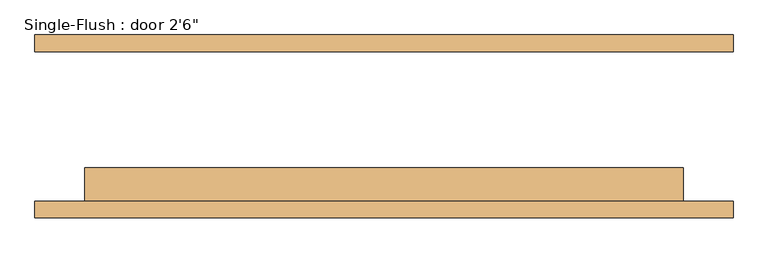
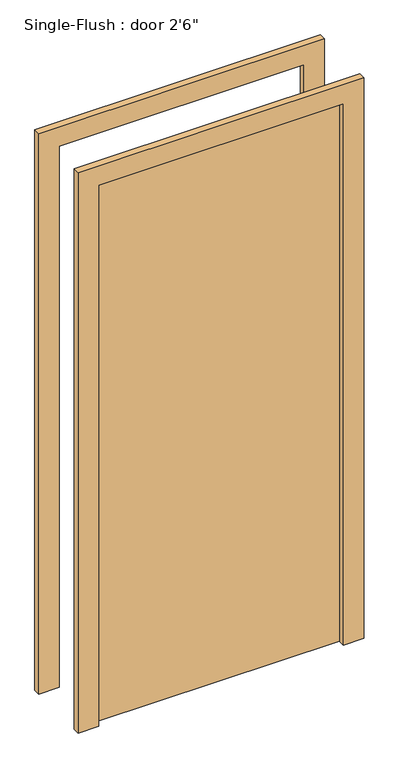
"""IFC4 building model written with IfcOpenShell, lengths in millimetres: door geometry."""

from ifc_helpers import new_model, si_unit, frame, origin, origin_with_axes, place, context, project, spatial, polyline, outline, extrude, source, transform, mapped, element, save


def door_a90ba1ad(model_context):
    return source(origin(), model_context, "Body", "SweptSolid", [
        extrude(outline(polyline([(2209.8, -533.4), (0.0, -533.4), (0.0, -457.2), (2133.6, -457.2), (2133.6, 457.2), (0.0, 457.2), (0.0, 533.4), (2209.8, 533.4), (2209.8, -533.4)])), frame((0.0, -139.7, 0.0), z_axis=(0.0, 1.0, 0.0), x_axis=(0.0, 0.0, 1.0)), (0.0, 0.0, 1.0), 25.4),
        extrude(outline(polyline([(2209.8, 533.4), (2209.8, -533.4), (0.0, -533.4), (0.0, -457.2), (2133.6, -457.2), (2133.6, 457.2), (0.0, 457.2), (0.0, 533.4), (2209.8, 533.4)])), frame((0.0, 114.3, 0.0), z_axis=(0.0, 1.0, 0.0), x_axis=(0.0, 0.0, 1.0)), (0.0, 0.0, 1.0), 25.4),
        extrude(outline(polyline([(457.2, -63.5), (457.2, -114.3), (-457.2, -114.3), (-457.2, -63.5), (457.2, -63.5)])), origin_with_axes(), (0.0, 0.0, 1.0), 2133.6),
    ])


if __name__ == "__main__":
    model = new_model("IFC4")
    model_context = context("Model", 3, world=origin())
    ifc_project = project(units=[si_unit("LENGTHUNIT", "METRE", prefix="MILLI")], contexts=[model_context])
    site = spatial("IfcSite", under=ifc_project)
    building = spatial("IfcBuilding", under=site)
    placement = place(None, origin())
    door_shape = door_a90ba1ad(model_context)
    element("IfcDoor", 1, ObjectType="Single-Flush : door 2'6\"", at=placement, inside=building, context=model_context, shape_type="MappedRepresentation", body=[
        mapped(door_shape, transform((0.0, 0.0, 0.0), x_axis=(1.0, 0.0, 0.0), y_axis=(0.0, 1.0, 0.0), z_axis=(0.0, 0.0, 1.0))),
    ])
    save(model, "model.ifc")

# Revit data of these elements
# Type "Single-Flush : door 2'6\""
#   Type Mark = "8"
#   Construction Type Id = "MDOOR"
#   Assembly Code = "C1020"
#   Analytic Construction = "Metal"
#   Thickness = 0' - 2"
#   Heat Transfer Coefficient (U) = 0.651978 BTU/(h·ft²·°F)
#   Height = 7' - 0"
#   Trim Projection Ext = 0' - 1"
#   Trim Projection Int = 0' - 1"
#   Trim Width = 0' - 3"
#   Width = 3' - 0"
#   Define Thermal Properties by = 1
#   Door Material = Door - Panel
#   Frame Material = Door - Frame
#   Visual Light Transmittance = 0
#   Solar Heat Gain Coefficient = 0
#   Function = (empty or 0)
#   Wall Closure = (empty or 0)
# Element 1 (IfcDoor, "Single-Flush : door 2'6\"")
#   Materials on its faces: "Door - Frame", "Door - Panel"
# Materials
#   "Door - Panel": class "Wood", colour RGB 210 159 95, transparency 0, Cost = 0
#   "Door - Frame": colour RGB 118 70 51, transparency 0, Cost = 0
